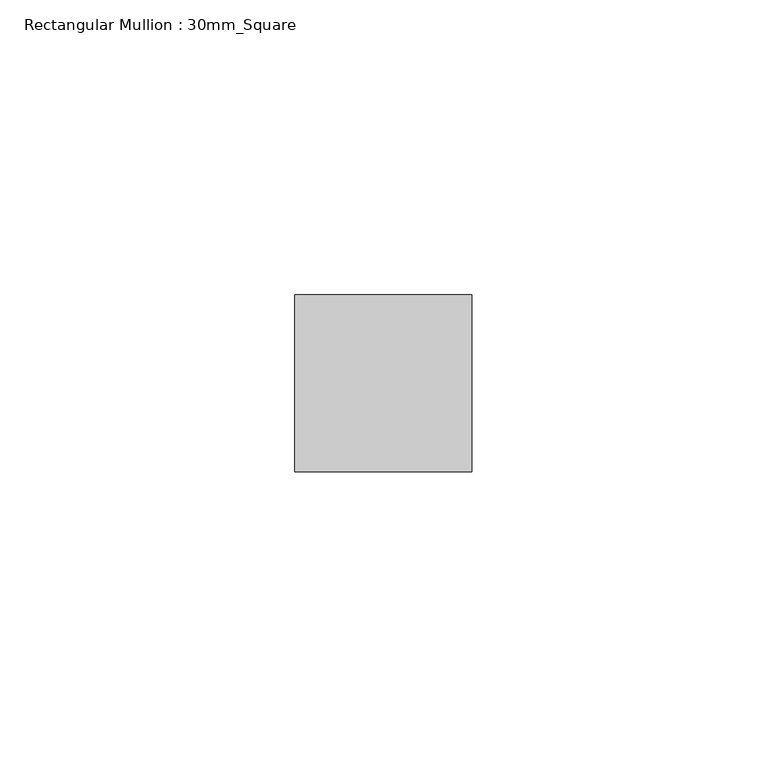
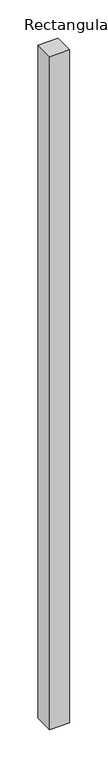
"""IFC4 building model written with IfcOpenShell, lengths in millimetres: member geometry, Rectangular Mullion : 30mm_Square."""

from ifc_helpers import new_model, si_unit, frame, origin, place, context, project, spatial, polyline, outline, extrude, source, transform, mapped, element, save


def rectangular_mullion_30mm_square_ca2d7245(model_context):
    return source(origin(), model_context, "Body", "SweptSolid", [
        extrude(outline(polyline([(15.0, 15.0), (15.0, -15.0), (-15.0, -15.0), (-15.0, 15.0), (15.0, 15.0)])), frame((0.0, 0.0, -1068.6296161), z_axis=(0.0, 0.0, 1.0), x_axis=(1.0, 0.0, 0.0)), (0.0, 0.0, 1.0), 1068.6296161),
    ])


if __name__ == "__main__":
    model = new_model("IFC4")
    model_context = context("Model", 3, world=origin())
    ifc_project = project(units=[si_unit("LENGTHUNIT", "METRE", prefix="MILLI")], contexts=[model_context])
    site = spatial("IfcSite", under=ifc_project)
    building = spatial("IfcBuilding", under=site)
    placement = place(None, origin())
    rectangular_mullion_30mm_square_shape = rectangular_mullion_30mm_square_ca2d7245(model_context)
    element("IfcMember", 1, ObjectType="Rectangular Mullion : 30mm_Square", at=placement, inside=building, context=model_context, shape_type="MappedRepresentation", body=[
        mapped(rectangular_mullion_30mm_square_shape, transform((0.0, 0.0, 0.0), x_axis=(1.0, 0.0, 0.0), y_axis=(0.0, 1.0, 0.0), z_axis=(0.0, 0.0, 1.0))),
    ])
    save(model, "model.ifc")

# Revit data of these elements
# Type "Rectangular Mullion : 30mm_Square"
#   Keynote = "H11"
#   built-in parameter 1007304 = 0.0984252 (stored number, unit not read)
#   built-in parameter 1007301 = 0.0492126 (stored number, unit not read)
#   built-in parameter 1007300 = 0.0492126 (stored number, unit not read)
# Element 1 (IfcMember, "Rectangular Mullion : 30mm_Square")
#   Materials on its faces: "Aluminium"
# Materials
#   "Aluminium": class "Metal", colour RGB 247 247 247, transparency 0, Description = "Aluminium 6061", Cost = 0
